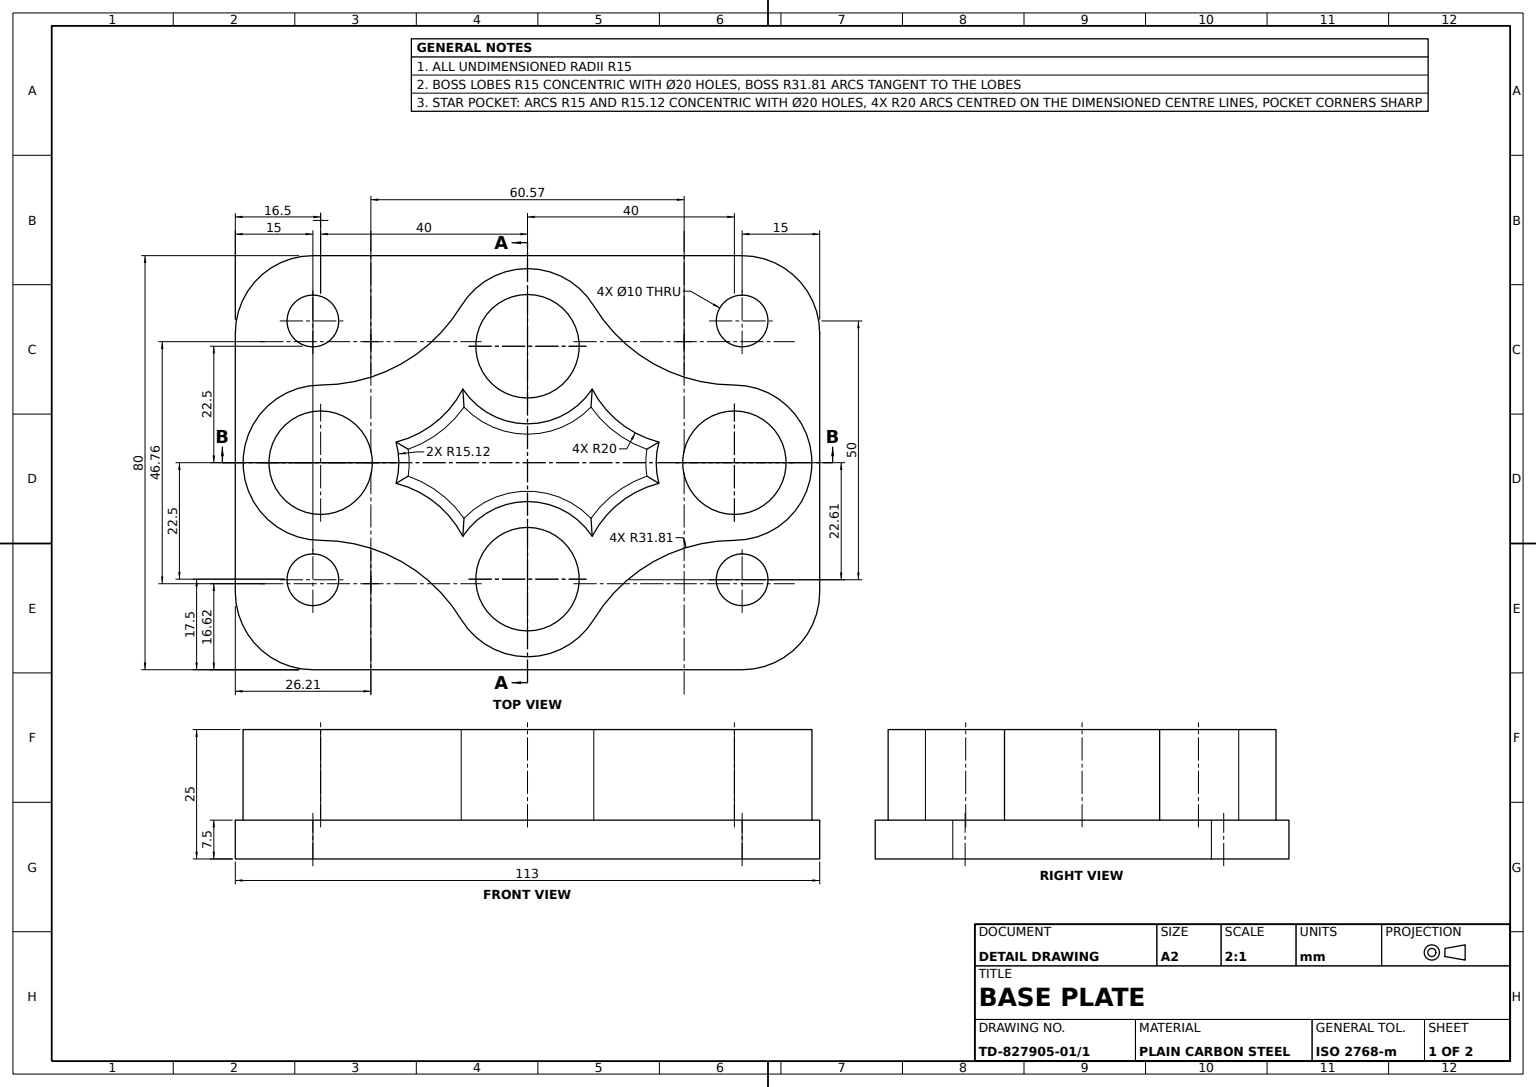
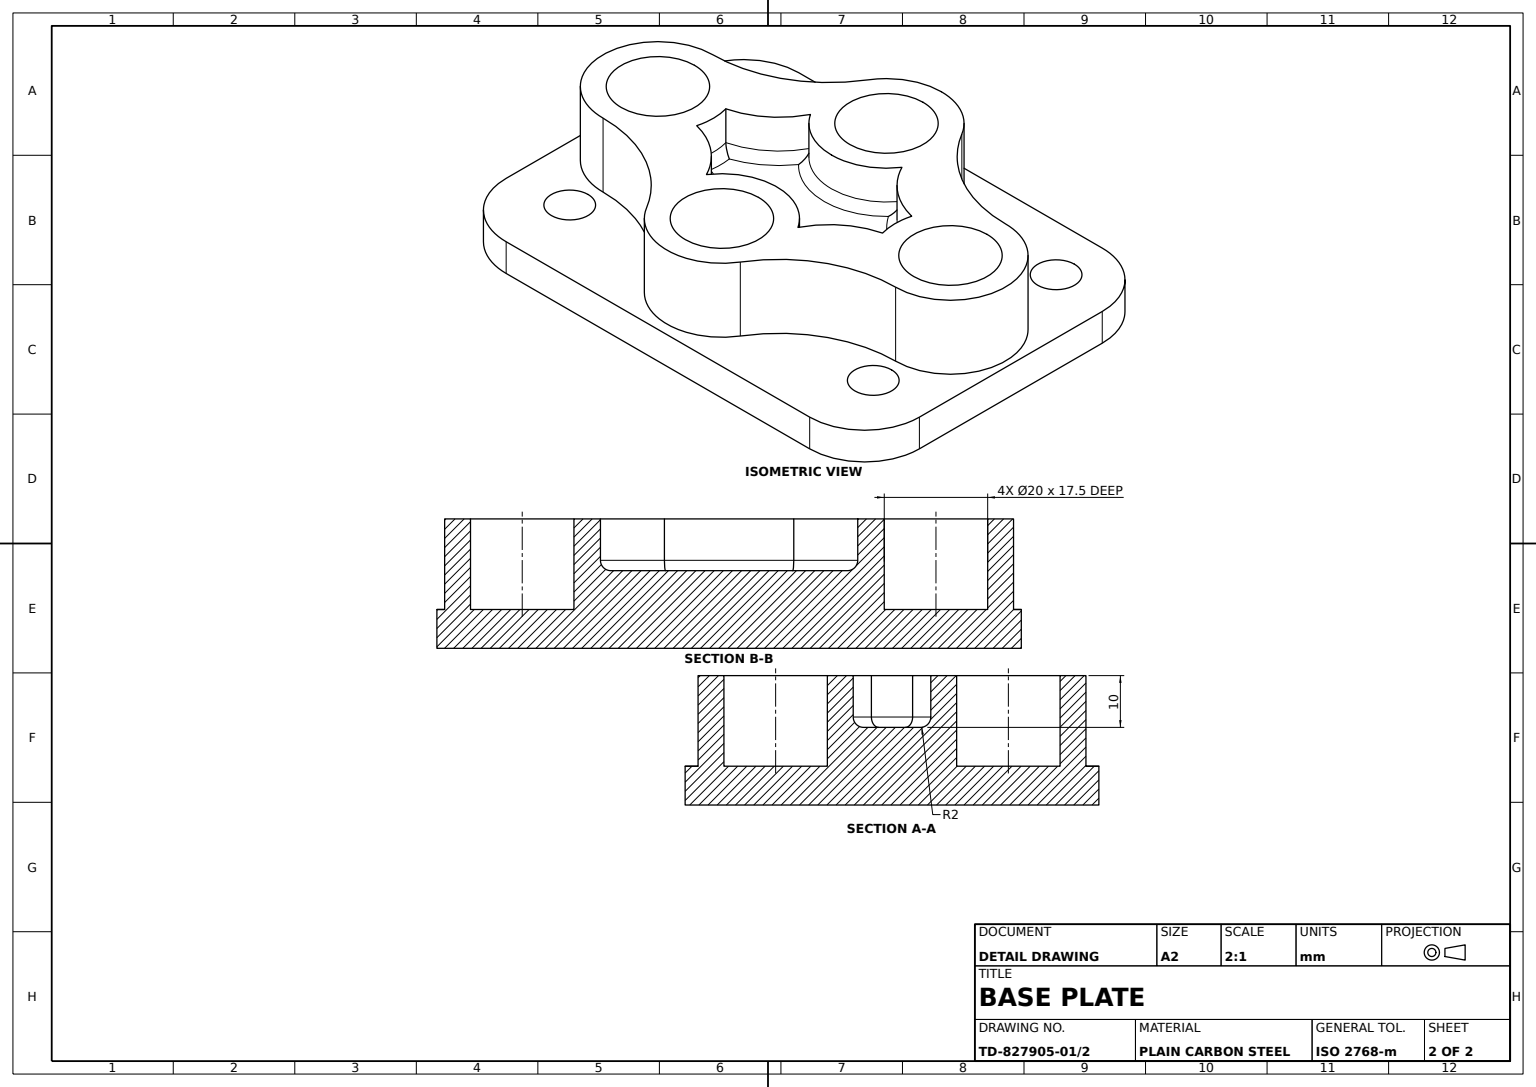
SolidWorks part; units mm, degrees
material "Plain Carbon Steel"
ref_plane "Front Plane" through (0, 0, 0) normal (0, 0, 1) x (1, 0, 0)
ref_plane "Top Plane" through (0, 0, 0) normal (0, 1, 0) x (1, 0, 0)
ref_plane "Right Plane" through (0, 0, 0) normal (1, 0, 0) x (0, 0, -1)
sketch "Base Plate Profile" plane through (0, 0, 0) normal (0, 1, 0) x (1, 0, 0)
  line L1 (41.5, -40) -> (-41.5, -40)
  line L2 (56.5, -25) -> (56.5, 25)
  line L3 (41.5, 40) -> (-41.5, 40)
  line L4 (-56.5, -25) -> (-56.5, 25)
  line L5 (56.5, -40) -> (-56.5, 40) construction
  line L6 (56.5, 40) -> (-56.5, -40) construction
  arc A0 (56.5, 25) -> (41.5, 40) centre (41.5, 25) ccw
  arc A1 (41.5, -40) -> (56.5, -25) centre (41.5, -25) ccw
  arc A2 (-41.5, -40) -> (-56.5, -25) centre (-41.5, -25) cw
  arc A3 (-41.5, 40) -> (-56.5, 25) centre (-41.5, 25) ccw
  point P0 (0, 0)
  dimension "D3" = 15
  dimension "D1" = 113
  dimension "D2" = 80
extrude "Base Plate" add sketch "Base Plate Profile" along normal mid plane 7.5
sketch "Mounting Holes Sketch" plane through (0, 3.75, 0) normal (0, 1, 0) x (1, 0, 0)
  line L0 (-56.5, 25) -> (-56.5, -25) construction
  line L1 (0, -13.75) -> (0, 13.75) construction
  circle A0 centre (-41.5, 27.3851) radius 5
  circle A1 centre (-41.5, -22.6149) radius 5
  circle A2 centre (41.5, -22.6149) radius 5
  circle A3 centre (41.5, 27.3851) radius 5
  dimension "D1" = 10
  dimension "D2" = 10
  dimension "D3" = 15
  dimension "D4" = 15
  dimension "D5" = 50
  dimension "D6" = 22.6149
extrude "Mounting Holes 4xØ10" cut sketch "Mounting Holes Sketch" against normal blind 7.5
sketch "Boss Layout Sketch" plane through (0, 3.75, 0) normal (0, 1, 0) x (1, 0, 0)
  line L0 (0, 22.5) -> (0, -22.5) construction
  line L1 (-40, 0) -> (40, 0) construction
  line L2 (-40, 19.4992) -> (-40, -28.8259) construction
  line L3 (-22.7734, 22.5) -> (24.4254, 22.5) construction
  circle A0 centre (0, 22.5) radius 10
  circle A1 centre (0, -22.5) radius 10
  circle A2 centre (-40, 0) radius 10
  circle A3 centre (40, 0) radius 10
  arc A4 (-40, 15) -> (-40, -15) centre (-40, 0) ccw
  arc A5 (-12.5078, 14.2202) -> (12.5078, 14.2202) centre (0, 22.5) ccw
  arc A6 (40, -15) -> (40, 15) centre (40, 0) ccw
  arc A7 (-12.819, -30.2893) -> (12.819, -30.2893) centre (0, -22.5) ccw
  arc A8 (-40, 15) -> (-12.819, 30.2893) centre (-40, 46.8056) ccw
  arc A9 (-25.4097, 3.9851) -> (-12.5078, 14.2202) centre (-30.2862, 23.3815) ccw
  arc A10 (-38.4027, 15.0401) -> (-38.4027, -15.0401) centre (-40, 0) ccw
  arc A11 (-25.4097, -3.9851) -> (-12.5078, -14.2202) centre (-30.2862, -23.3815) cw
  arc A12 (25.4097, -3.9851) -> (12.5078, -14.2202) centre (30.2862, -23.3815) ccw
  arc A13 (25.4097, 3.9851) -> (12.5078, 14.2202) centre (30.2862, 23.3815) cw
  arc A14 (-40, -15) -> (-12.819, -30.2893) centre (-40, -46.8056) cw
  arc A15 (40, -15) -> (12.819, -30.2893) centre (40, -46.8056) ccw
  arc A16 (40, 15) -> (12.819, 30.2893) centre (40, 46.8056) cw
  arc A17 (-25.4097, -3.9851) -> (-25.4097, 3.9851) centre (-40, 0) ccw
  arc A18 (12.5078, -14.2202) -> (-12.5078, -14.2202) centre (0, -22.5) ccw
  arc A19 (25.4097, -3.9851) -> (25.4097, 3.9851) centre (40, 0) cw
  arc A20 (12.819, 30.2893) -> (-12.819, 30.2893) centre (0, 22.5) ccw
  point P4 (0, 0)
  point P10 (0, 0)
  dimension "D1" = 20
  dimension "D2" = 20
  dimension "D3" = 20
  dimension "D4" = 20
  dimension "D5" = 30
  dimension "D6" = 20
  dimension "D7" = 31.8056
  dimension "D8" = 15.1247
  dimension "D9" = 16.5
  dimension "D10" = 26.2138
  dimension "D11" = 31.0903
sketch "Lobed Boss Profile" plane through (0, 3.75, 0) normal (0, 1, 0) x (1, 0, 0)
  arc A0 (-40, 15) -> (-40, -15) centre (-40, 0) ccw construction
  arc A1 (-12.819, -30.2893) -> (-40, -15) centre (-40, -46.8056) ccw construction
  arc A2 (-12.819, -30.2893) -> (12.819, -30.2893) centre (0, -22.5) ccw construction
  arc A3 (40, -15) -> (12.819, -30.2893) centre (40, -46.8056) ccw construction
  arc A4 (40, -15) -> (40, 15) centre (40, 0) ccw construction
  arc A5 (12.819, 30.2893) -> (40, 15) centre (40, 46.8056) ccw construction
  arc A6 (12.819, 30.2893) -> (-12.819, 30.2893) centre (0, 22.5) ccw construction
  arc A7 (-40, 15) -> (-12.819, 30.2893) centre (-40, 46.8056) ccw construction
  arc A8 (-40, 15) -> (-40, -15) centre (-40, 0) ccw
  arc A9 (-12.819, -30.2893) -> (-40, -15) centre (-40, -46.8056) ccw
  arc A10 (-12.819, -30.2893) -> (12.819, -30.2893) centre (0, -22.5) ccw
  arc A11 (40, -15) -> (12.819, -30.2893) centre (40, -46.8056) ccw
  arc A12 (40, -15) -> (40, 15) centre (40, 0) ccw
  arc A13 (12.819, 30.2893) -> (40, 15) centre (40, 46.8056) ccw
  arc A14 (12.819, 30.2893) -> (-12.819, 30.2893) centre (0, 22.5) ccw
  arc A15 (-40, 15) -> (-12.819, 30.2893) centre (-40, 46.8056) ccw
extrude "Lobed Boss" add sketch "Lobed Boss Profile" along normal blind 17.5
sketch "Star Pocket Profile" plane through (0, 21.25, 0) normal (0, 1, 0) x (1, 0, 0)
  arc A0 (-25.4097, -3.9851) -> (-25.4097, 3.9851) centre (-40, 0) ccw construction
  arc A1 (-12.5078, -14.2202) -> (-25.4097, -3.9851) centre (-30.2862, -23.3815) ccw construction
  arc A2 (12.5078, -14.2202) -> (-12.5078, -14.2202) centre (0, -22.5) ccw construction
  arc A3 (25.4097, -3.9851) -> (12.5078, -14.2202) centre (30.2862, -23.3815) ccw construction
  arc A4 (25.4097, 3.9851) -> (25.4097, -3.9851) centre (40, 0) ccw construction
  arc A5 (12.5078, 14.2202) -> (25.4097, 3.9851) centre (30.2862, 23.3815) ccw construction
  arc A6 (-12.5078, 14.2202) -> (12.5078, 14.2202) centre (0, 22.5) ccw construction
  arc A7 (-25.4097, 3.9851) -> (-12.5078, 14.2202) centre (-30.2862, 23.3815) ccw construction
  arc A8 (-25.4097, -3.9851) -> (-25.4097, 3.9851) centre (-40, 0) ccw
  arc A9 (-12.5078, -14.2202) -> (-25.4097, -3.9851) centre (-30.2862, -23.3815) ccw
  arc A10 (12.5078, -14.2202) -> (-12.5078, -14.2202) centre (0, -22.5) ccw
  arc A11 (25.4097, -3.9851) -> (12.5078, -14.2202) centre (30.2862, -23.3815) ccw
  arc A12 (25.4097, 3.9851) -> (25.4097, -3.9851) centre (40, 0) ccw
  arc A13 (12.5078, 14.2202) -> (25.4097, 3.9851) centre (30.2862, 23.3815) ccw
  arc A14 (-12.5078, 14.2202) -> (12.5078, 14.2202) centre (0, 22.5) ccw
  arc A15 (-25.4097, 3.9851) -> (-12.5078, 14.2202) centre (-30.2862, 23.3815) ccw
extrude "Star Pocket" cut sketch "Star Pocket Profile" against normal blind 10
sketch "Boss Bores Sketch" plane through (0, 21.25, 0) normal (0, 1, 0) x (1, 0, 0)
  circle A0 centre (40, 0) radius 10 construction
  circle A1 centre (0, -22.5) radius 10 construction
  circle A2 centre (0, 22.5) radius 10 construction
  circle A3 centre (-40, 0) radius 10 construction
  circle A4 centre (40, 0) radius 10
  circle A5 centre (0, -22.5) radius 10
  circle A6 centre (0, 22.5) radius 10
  circle A7 centre (-40, 0) radius 10
extrude "Boss Bores 4x" cut sketch "Boss Bores Sketch" against normal blind 17.5
fillet "Pocket Fillets R2" radius 2 8 edges at (-17.8564, 11.25, 7.7131) (0, 11.25, 7.5) (17.8564, 11.25, 7.7131) (-17.8564, 11.25, -7.7131) (0, 11.25, -7.5) (17.8564, 11.25, -7.7131) (-24.8753, 11.25, 0) (24.8753, 11.25, 0)
